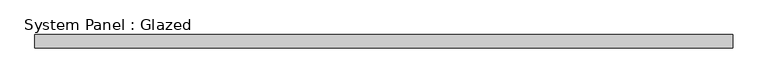
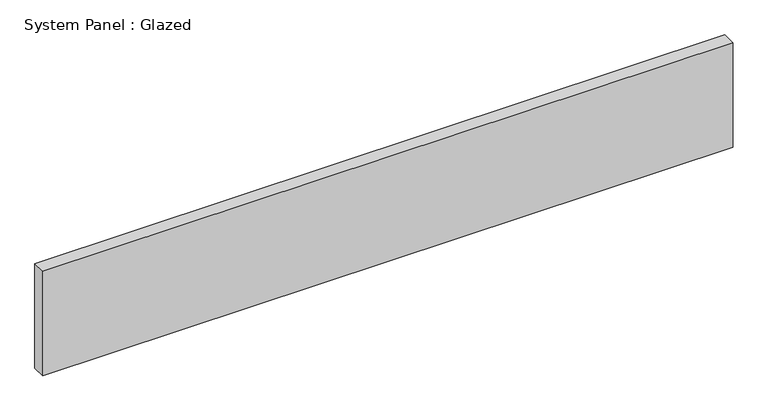
"""IFC4 building model written with IfcOpenShell, lengths in millimetres: plate geometry, System Panel : Glazed."""

from ifc_helpers import new_model, si_unit, origin, origin_with_axes, place, context, project, spatial, polyline, outline, extrude, source, transform, mapped, element, save


def system_panel_glazed_ad1fd27a(model_context):
    return source(origin(), model_context, "Body", "SweptSolid", [
        extrude(outline(polyline([(654.05, 19.05), (-654.05, 19.05), (-654.05, 44.45), (654.05, 44.45), (654.05, 19.05)])), origin_with_axes(), (0.0, 0.0, 1.0), 209.55),
    ])


if __name__ == "__main__":
    model = new_model("IFC4")
    model_context = context("Model", 3, world=origin())
    ifc_project = project(units=[si_unit("LENGTHUNIT", "METRE", prefix="MILLI")], contexts=[model_context])
    site = spatial("IfcSite", under=ifc_project)
    building = spatial("IfcBuilding", under=site)
    placement = place(None, origin())
    system_panel_glazed_shape = system_panel_glazed_ad1fd27a(model_context)
    element("IfcPlate", 1, ObjectType="System Panel : Glazed", at=placement, inside=building, context=model_context, shape_type="MappedRepresentation", body=[
        mapped(system_panel_glazed_shape, transform((0.0, 0.0, 0.0), x_axis=(1.0, 0.0, 0.0), y_axis=(0.0, 1.0, 0.0), z_axis=(0.0, 0.0, 1.0))),
    ])
    save(model, "model.ifc")

# Revit data of these elements
# Type "System Panel : Glazed"
#   Construction Type Id = "GSP4R"
#   Analytic Construction = "1/8 in Pilkington single glazing"
#   Visual Light Transmittance = 0.9
#   Solar Heat Gain Coefficient = 0.86
#   Heat Transfer Coefficient (U) = 1.18115 BTU/(h·ft²·°F)
#   Define Thermal Properties by = 1
# Element 1 (IfcPlate, "System Panel : Glazed")
#   Materials on its faces: "Glass"
# Materials
#   "Glass": class "Glass", colour RGB 0 128 192, transparency 0.75, Description = "Soda Lime Glass", Cost = 0
